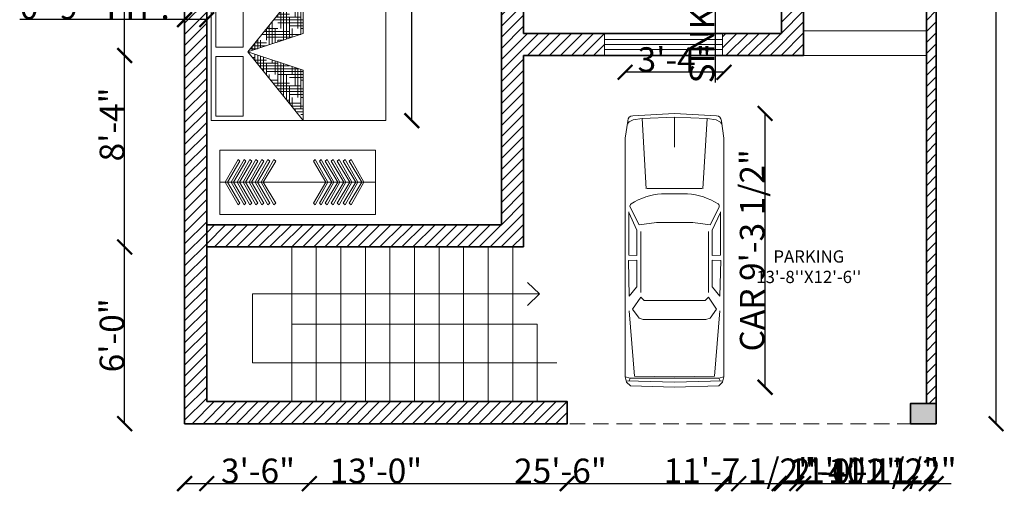
# Model space of a CAD drawing. Units: inches. Extents: x 1957 to 2456, y 1504 to 2088.
# Tile 1 of 6: x 1998 to 2399, y 1504 to 1703. Entities that reach past the tile are written whole.
import ezdxf

# ---------------------------------------------------------------- set-up
doc = ezdxf.new("R2010")
doc.units = ezdxf.units.IN
doc.header["$LTSCALE"] = 2
doc.linetypes.add('HIDDEN2', pattern=[4.7625, 3.175, -1.5875])
for name, color, linetype, lineweight in [('A-ANNO-DIMS', 2, 'Continuous', 18), ('A-ANNO-SYMB', 50, 'Continuous', 18), ('A-AREA-IDEN', 7, 'Continuous', 18), ('A-COLS', 12, 'Continuous', 35), ('A-COLS-PATT', 12, 'Continuous', 13), ('A-EQPM-VEHI', 8, 'Continuous', 18), ('A-FURN', 8, 'Continuous', 18), ('A-WALL-HIDN', 7, 'HIDDEN2', 18), ('A-WALL-PATT', 8, 'Continuous', 13), ('shelves', 204, 'Continuous', 18), ('Steps', 50, 'Continuous', 18), ('Walls', 7, 'Continuous', 35), ('Windows', 140, 'Continuous', 18)]:
    doc.layers.add(name, color=color, linetype=linetype, lineweight=lineweight)
doc.styles.get("Standard").update_dxf_attribs({"font": 'arial.ttf'})
doc.dimstyles.get("Standard").update_dxf_attribs({"dimtxt": 10, "dimasz": 6, "dimexe": 0.18, "dimexo": 0.0625, "dimgap": 0.09, "dimtad": 1, "dimdec": 1, "dimzin": 0, "dimdsep": 46, "dimlunit": 4, "dimtxsty": 'Standard', "dimblk": 'ARCHTICK', "dimcen": 0.09, "dimse1": 1, "dimse2": 1, "dimadec": 0, "dimazin": 0, "dimtfac": 1, "dimtdec": 1, "dimtofl": 0, "dimtmove": 0, "dimatfit": 3, "dimfxl": 1, "dimtolj": 1, "dimtzin": 0, "dimarcsym": 0})

# ---------------------------------------------------------------- blocks, each defined once
blk = doc.blocks.new('*X4')
at = {"color": 0}
for p, q in [((20.25, 14.812), (20.277, 14.812)), ((20.124, 14.688), (20.25, 14.688)), ((20.125, 14.5), (20.125, 14.689)), ((20.149, 14.719), (20.277, 14.719)), ((20.156, 14.625), (20.156, 14.728)), ((20.174, 14.75), (20.277, 14.75)), ((20.188, 14.75), (20.188, 14.767)), ((20.199, 14.781), (20.277, 14.781)), ((20.25, 14.319), (20.25, 14.75)), ((20.062, 14.257), (20.062, 14.612)), ((20.094, 14.375), (20.094, 14.65)), ((20.098, 14.656), (20.125, 14.656)), ((20.125, 14.594), (20.277, 14.594)), ((20.219, 14.309), (20.219, 14.625)), ((20.25, 14.625), (20.277, 14.625)), ((19.973, 14.5), (20.25, 14.5)), ((19.998, 14.531), (20.277, 14.531)), ((20, 14.237), (20, 14.5)), ((20.023, 14.562), (20.277, 14.562)), ((20.031, 14.247), (20.031, 14.573)), ((20.188, 14.299), (20.188, 14.5)), ((19.875, 14.25), (19.875, 14.379)), ((19.906, 14.375), (19.906, 14.417)), ((19.922, 14.438), (20, 14.438)), ((19.948, 14.469), (20.125, 14.469)), ((19.969, 14.226), (19.969, 14.375)), ((20, 14.375), (20.277, 14.375)), ((20.125, 14.406), (20.277, 14.406)), ((20.156, 14.288), (20.156, 14.375)), ((20.25, 14.438), (20.277, 14.438)), ((19.781, 14.164), (19.781, 14.262)), ((19.797, 14.281), (20.125, 14.281)), ((19.812, 14.174), (19.812, 14.301)), ((19.822, 14.312), (20.229, 14.312)), ((19.844, 14.185), (19.844, 14.34)), ((19.875, 14.344), (20.277, 14.344)), ((19.721, 14.188), (19.75, 14.188)), ((19.746, 14.219), (19.875, 14.219)), ((19.75, 14.154), (19.75, 14.223)), ((19.772, 14.25), (20, 14.25)), ((19.938, 14.216), (19.938, 14.25)), ((19.702, 14.094), (19.779, 14.094)), ((19.719, 14.073), (19.719, 14.114)), ((19.727, 14.062), (19.873, 14.062)), ((19.75, 14.034), (19.75, 14.103)), ((19.781, 13.995), (19.781, 14.093)), ((19.812, 14), (19.812, 14.082)), ((19.906, 13.84), (19.906, 14.051)), ((19.752, 14.031), (19.875, 14.031)), ((19.827, 13.938), (20.25, 13.938)), ((19.875, 13.878), (19.875, 14)), ((19.875, 13.969), (20.156, 13.969)), ((19.938, 13.801), (19.938, 14.041)), ((19.969, 13.875), (19.969, 14.031)), ((20, 14), (20, 14.02)), ((20, 14), (20.061, 14)), ((20.062, 13.645), (20.062, 14)), ((20.094, 13.625), (20.094, 13.989)), ((20.125, 13.75), (20.125, 13.979)), ((20.156, 13.875), (20.156, 13.969)), ((20.25, 13.5), (20.25, 13.937)), ((19.853, 13.906), (20.125, 13.906)), ((19.878, 13.875), (20, 13.875)), ((20.031, 13.684), (20.031, 13.875)), ((20.125, 13.844), (20.277, 13.844)), ((20.219, 13.451), (20.219, 13.875)), ((20.25, 13.875), (20.277, 13.875)), ((19.953, 13.781), (20.277, 13.781)), ((19.978, 13.75), (20.25, 13.75)), ((20, 13.812), (20.277, 13.812)), ((20, 13.723), (20, 13.75)), ((20.188, 13.49), (20.188, 13.75)), ((20.003, 13.719), (20.125, 13.719)), ((20.079, 13.625), (20.277, 13.625)), ((20.125, 13.656), (20.277, 13.656)), ((20.156, 13.529), (20.156, 13.625)), ((20.25, 13.688), (20.277, 13.688)), ((20.104, 13.594), (20.277, 13.594)), ((20.129, 13.562), (20.25, 13.562)), ((20.205, 13.469), (20.277, 13.469)), ((20.23, 13.438), (20.277, 13.438)), ((20.25, 13.5), (20.277, 13.5)), ((20.255, 13.406), (20.277, 13.406))]:
    blk.add_line(p, q, dxfattribs=at)
blk = doc.blocks.new('MAT-P13')
for p, q in [((-0.75, 0), (0.75, 0)), ((-0.75, 0), (-0.75, -1.9)), ((0.75, 0), (0.75, -1.9)), ((-0.7, -0.05), (-0.7, -0.35)), ((-0.7, -0.05), (-0.05, -0.05)), ((-0.05, -0.35), (-0.05, -0.05)), ((0.05, -0.05), (0.7, -0.05)), ((0.05, -0.35), (0.05, -0.05)), ((0.7, -0.05), (0.7, -0.35)), ((-0.75, -1.003), (0, -0.4)), ((0, -0.4), (-0.75, -1.003)), ((-0.7, -0.35), (-0.05, -0.35)), ((0, -0.4), (-0.2, -1.003)), ((0, -0.4), (0.2, -1.003)), ((0, -0.4), (0.75, -1.003)), ((0.05, -0.35), (0.7, -0.35)), ((-0.75, -1.003), (-0.2, -1.003)), ((0.2, -1.003), (0.75, -1.003)), ((0.75, -1.9), (-0.75, -1.9))]:
    blk.add_line(p, q)
at = {"xscale": -1, "rotation": 90}
blk.add_blockref('*X4', (14.128, 19.274), dxfattribs=at)
blk = doc.blocks.new('02PCAR12')
at = {"color": 0, "linetype": 'ByBlock'}
for p, q in [((-203, 38), (-207, 37)), ((-203, 38.08), (-204, 34.08)), ((-19, 38), (-203, 38)), ((-6, 36), (-19, 38)), ((-210, 34), (-211, 0)), ((-207, 37), (-210, 34)), ((-206, 37), (-207, 0)), ((-204, 34.08), (-206, 35.08)), ((-204, -34), (-204, 34)), ((-202.36, 30.78), (-203, 0)), ((-202.36, 30.78), (-152, 35)), ((-150.83, 32.3), (-157.9, 27.3)), ((-141.48, 25.99), (-150.83, 32.3)), ((-113.23, 35.5), (-140.79, 34.89)), ((-140.79, 34.89), (-133.96, 29.23)), ((-113, 29), (-113.23, 35.5)), ((-109.42, 29.02), (-109.19, 35.33)), ((-109.19, 35.33), (-75.91, 35.3)), ((-76.45, 35.3), (-90, 29)), ((-72.15, 34.24), (-85.91, 27.37)), ((-5, 32), (-6.45, 34.89)), ((-5, 32), (-4, 25)), ((0, 0), (-1.8, 32.21)), ((-157.9, 27.3), (-158.93, 24.08)), ((-158.93, 24.08), (-158.93, -24)), ((-141.48, 25.99), (-144.24, 23.52)), ((-144.24, 23.52), (-144.24, 0)), ((-91, 26), (-138, 26)), ((-134, 29), (-113, 29)), ((-90, 29), (-109.42, 29.02)), ((-58.25, 21.76), (-4, 25)), ((-4, 25), (-3, 0)), ((-58, 0), (-58, 21)), ((-84, -12), (-84, 12)), ((-62, 10), (-62, 0)), ((-210, -34), (-211, 0)), ((-206, -37), (-207, 0)), ((-202.36, -30.78), (-203, 0)), ((-144.24, -23.52), (-144.24, 0)), ((-62, -10), (-62, 0)), ((-58, 0), (-58, -21)), ((-3, 0), (-26, 0)), ((-4, -25), (-3, 0)), ((0, 0), (-1.8, -32.21)), ((-58.25, -21.76), (-4, -25)), ((-157.9, -27.3), (-158.93, -24.08)), ((-150.83, -32.3), (-157.9, -27.3)), ((-141.48, -25.99), (-150.83, -32.3)), ((-141.48, -25.99), (-144.24, -23.52)), ((-140.79, -34.89), (-133.96, -29.23)), ((-91, -26), (-138, -26)), ((-134, -29), (-113, -29)), ((-113, -29), (-113.23, -35.5)), ((-90, -29), (-109.42, -29.02)), ((-109.42, -29.02), (-109.19, -35.33)), ((-76.45, -35.3), (-90, -29)), ((-72.15, -34.24), (-85.91, -27.37)), ((-5, -32), (-4, -25)), ((-207, -37), (-210, -34)), ((-203, -38), (-207, -37)), ((-204, -34), (-206, -35)), ((-203, -38), (-204, -34)), ((-202.36, -30.69), (-152, -34.92)), ((-113.23, -35.5), (-140.79, -34.89)), ((-109.19, -35.33), (-75.91, -35.3)), ((-6, -36), (-19, -38)), ((-5, -32), (-6.45, -34.89)), ((-19, -38), (-203, -38))]:
    blk.add_line(p, q, dxfattribs=at)
for centre, radius, start, end in [((-71.36, 32.4), 2, 31.5638, 113.12574), ((-115.33, 5.39), 53.61, 4.93792, 31.5638), ((-8.24, 34), 2, 26.56505, 90), ((-5.8, 32), 4, 3.01279, 90), ((-461.05, -27.14), 379.08, 5.92644, 8.26698), ((-461.05, 27.14), 379.08, 351.73302, 354.07356), ((-115.33, -5.39), 53.61, 328.4362, 355.06208), ((-71.36, -32.4), 2, 246.87426, 328.4362), ((-8.24, -34), 2, 270, 333.43495), ((-5.8, -32), 4, 270, 356.98721)]:
    blk.add_arc(centre, radius, start, end, dxfattribs=at)
blk = doc.blocks.new('WIN-48IN')
for p, q in [((0, 6.5), (48, 6.5)), ((0, 4.5), (48, 4.5)), ((0, 2.5), (48, 2.5))]:
    blk.add_line(p, q)
blk.add_lwpolyline([(0, 9), (48, 9), (48, 0), (0, 0)], close=True)
blk = doc.blocks.new('WARDROBE-RAIL')
blk.add_line((0, 13.12), (63.46, 13.12))
blk.add_lwpolyline([(0, 26.23), (63.46, 26.23), (63.46, 0), (0, 0)], close=True)
for points in [[(2.25, 13.12), (7.43, 22.31), (8.16, 21.63), (3.1, 13.12)], [(4.68, 13.12), (9.87, 22.31), (10.6, 21.63), (5.54, 13.12)], [(7.12, 13.12), (12.3, 22.31), (13.03, 21.63), (7.98, 13.12)], [(9.56, 13.12), (14.74, 22.31), (15.47, 21.63), (10.41, 13.12)], [(11.99, 13.12), (17.18, 22.31), (17.91, 21.63), (12.85, 13.12)], [(14.43, 13.12), (19.61, 22.31), (20.34, 21.63), (15.29, 13.12)], [(16.87, 13.12), (22.05, 22.31), (22.78, 21.63), (17.72, 13.12)], [(44.01, 13.12), (38.82, 22.31), (38.09, 21.63), (43.15, 13.12)], [(46.44, 13.12), (41.26, 22.31), (40.53, 21.63), (45.59, 13.12)], [(48.88, 13.12), (43.7, 22.31), (42.96, 21.63), (48.02, 13.12)], [(51.31, 13.12), (46.13, 22.31), (45.4, 21.63), (50.46, 13.12)], [(53.75, 13.12), (48.57, 22.31), (47.84, 21.63), (52.89, 13.12)], [(56.19, 13.12), (51.01, 22.31), (50.27, 21.63), (55.33, 13.12)], [(58.62, 13.12), (53.44, 22.31), (52.71, 21.63), (57.77, 13.12)], [(2.25, 13.12), (7.43, 3.92), (8.16, 4.61), (3.1, 13.12)], [(4.68, 13.12), (9.87, 3.92), (10.6, 4.61), (5.54, 13.12)], [(7.12, 13.12), (12.3, 3.92), (13.03, 4.61), (7.98, 13.12)], [(9.56, 13.12), (14.74, 3.92), (15.47, 4.61), (10.41, 13.12)], [(11.99, 13.12), (17.18, 3.92), (17.91, 4.61), (12.85, 13.12)], [(14.43, 13.12), (19.61, 3.92), (20.34, 4.61), (15.29, 13.12)], [(16.87, 13.12), (22.05, 3.92), (22.78, 4.61), (17.72, 13.12)], [(44.01, 13.12), (38.82, 3.92), (38.09, 4.61), (43.15, 13.12)], [(46.44, 13.12), (41.26, 3.92), (40.53, 4.61), (45.59, 13.12)], [(48.88, 13.12), (43.7, 3.92), (42.96, 4.61), (48.02, 13.12)], [(51.31, 13.12), (46.13, 3.92), (45.4, 4.61), (50.46, 13.12)], [(53.75, 13.12), (48.57, 3.92), (47.84, 4.61), (52.89, 13.12)], [(56.19, 13.12), (51.01, 3.92), (50.27, 4.61), (55.33, 13.12)], [(58.62, 13.12), (53.44, 3.92), (52.71, 4.61), (57.77, 13.12)]]:
    blk.add_lwpolyline(points)
blk = doc.blocks.new('_ArchTick')
at = {"color": 0, "linetype": 'ByBlock', "const_width": 0.15}
blk.add_lwpolyline([(-0.5, -0.5), (0.5, 0.5)], dxfattribs=at)
blk = doc.blocks.new('*D24')
at = {"layer": 'A-ANNO-DIMS', "color": 0, "lineweight": -2, "transparency": 16777216}
for p, q in [((2065.03, 1702.85), (1997.9, 1702.85)), ((2074.03, 1702.85), (2065.03, 1702.85))]:
    blk.add_line(p, q, dxfattribs=at)
at = {"layer": 'Defpoints', "color": 0, "transparency": 16777216}
for p in [(2065.03, 1710.05), (2074.03, 1710.05), (2065.03, 1702.85)]:
    blk.add_point(p, dxfattribs=at)
at = {"layer": 'A-ANNO-DIMS', "color": 0, "lineweight": -2, "transparency": 16777216, "xscale": 6, "yscale": 6, "zscale": 6}
for p, rotation in [((2065.03, 1702.85), 179.9999999999986), ((2074.03, 1702.85), 359.9999999999986)]:
    blk.add_blockref('_ArchTick', p, dxfattribs=dict(at, rotation=rotation))
at = {"layer": 'A-ANNO-DIMS', "color": 0, "transparency": 16777216, "insert": (2028.47, 1708.05), "char_height": 10, "attachment_point": 5}
blk.add_mtext('\\A1;0\'-9" TYP.', dxfattribs=at)
blk = doc.blocks.new('*D30')
at = {"layer": 'A-ANNO-DIMS', "color": 0, "lineweight": -2, "transparency": 16777216}
for p, q in [((2157.56, 1717.76), (2157.56, 1785.3)), ((2157.56, 1661.68), (2157.56, 1717.76))]:
    blk.add_line(p, q, dxfattribs=at)
at = {"layer": 'Defpoints', "color": 0, "transparency": 16777216}
for p in [(2146.9, 1717.76), (2157.56, 1717.76), (2146.9, 1661.68)]:
    blk.add_point(p, dxfattribs=at)
at = {"layer": 'A-ANNO-DIMS', "color": 0, "lineweight": -2, "transparency": 16777216, "xscale": 6, "yscale": 6, "zscale": 6}
for p, rotation in [((2157.56, 1717.76), 90), ((2157.56, 1661.68), 270)]:
    blk.add_blockref('_ArchTick', p, dxfattribs=dict(at, rotation=rotation))
at = {"layer": 'A-ANNO-DIMS', "color": 0, "transparency": 16777216, "insert": (2152.36, 1754.53), "char_height": 10, "attachment_point": 5, "rotation": 90}
blk.add_mtext('\\A1;4\'-8" TYP.', dxfattribs=at)
blk = doc.blocks.new('*D41')
at = {"layer": 'A-ANNO-DIMS', "color": 0, "lineweight": -2, "transparency": 16777216}
for p, q in [((2281, 1801.1), (2281, 1777.56)), ((2281, 1777.56), (2281, 1677.29))]:
    blk.add_line(p, q, dxfattribs=at)
at = {"layer": 'Defpoints', "color": 0, "transparency": 16777216}
for p in [(2284.53, 1801.1), (2281, 1777.56), (2284.53, 1777.56)]:
    blk.add_point(p, dxfattribs=at)
at = {"layer": 'A-ANNO-DIMS', "color": 0, "lineweight": -2, "transparency": 16777216, "xscale": 6, "yscale": 6, "zscale": 6}
for p, rotation in [((2281, 1801.1), 90), ((2281, 1777.56), 270)]:
    blk.add_blockref('_ArchTick', p, dxfattribs=dict(at, rotation=rotation))
at = {"layer": 'A-ANNO-DIMS', "color": 0, "transparency": 16777216, "insert": (2275.74, 1724.42), "char_height": 10, "attachment_point": 5, "rotation": 90}
blk.add_mtext('\\A1;SINK 1\'-11 1/2"', dxfattribs=at)
blk = doc.blocks.new('*D43')
at = {"layer": 'A-ANNO-DIMS', "color": 0, "lineweight": -2, "transparency": 16777216}
blk.add_line((2301.35, 1553.07), (2301.35, 1664.66), dxfattribs=at)
at = {"layer": 'Defpoints', "color": 0, "transparency": 16777216}
for p in [(2284.62, 1664.66), (2301.35, 1664.66), (2284.62, 1553.07)]:
    blk.add_point(p, dxfattribs=at)
at = {"layer": 'A-ANNO-DIMS', "color": 0, "lineweight": -2, "transparency": 16777216, "xscale": 6, "yscale": 6, "zscale": 6}
for p, rotation in [((2301.35, 1664.66), 90), ((2301.35, 1553.07), 270)]:
    blk.add_blockref('_ArchTick', p, dxfattribs=dict(at, rotation=rotation))
at = {"layer": 'A-ANNO-DIMS', "color": 0, "transparency": 16777216, "insert": (2296.09, 1608.86), "char_height": 10, "attachment_point": 5, "rotation": 90}
blk.add_mtext('\\A1;CAR 9\'-3 1/2"', dxfattribs=at)
blk = doc.blocks.new('*D44')
at = {"layer": 'A-ANNO-DIMS', "color": 0, "lineweight": -2, "transparency": 16777216}
blk.add_line((2284.62, 1681.39), (2244.38, 1681.39), dxfattribs=at)
at = {"layer": 'Defpoints', "color": 0, "transparency": 16777216}
for p in [(2244.38, 1681.39), (2244.38, 1664.66), (2284.62, 1664.66)]:
    blk.add_point(p, dxfattribs=at)
at = {"layer": 'A-ANNO-DIMS', "color": 0, "lineweight": -2, "transparency": 16777216, "xscale": 6, "yscale": 6, "zscale": 6, "rotation": 180}
blk.add_blockref('_ArchTick', (2244.38, 1681.39), dxfattribs=at)
at = {"layer": 'A-ANNO-DIMS', "color": 0, "lineweight": -2, "transparency": 16777216, "xscale": 6, "yscale": 6, "zscale": 6}
blk.add_blockref('_ArchTick', (2284.62, 1681.39), dxfattribs=at)
at = {"layer": 'A-ANNO-DIMS', "color": 0, "transparency": 16777216, "insert": (2264.5, 1686.59), "char_height": 10, "attachment_point": 5}
blk.add_mtext('\\A1;3\'-4"', dxfattribs=at)
blk = doc.blocks.new('*D45')
at = {"layer": 'A-ANNO-DIMS', "color": 0, "lineweight": -2, "transparency": 16777216}
blk.add_line((2065.03, 1513.82), (2371.03, 1513.82), dxfattribs=at)
at = {"layer": 'Defpoints', "color": 0, "transparency": 16777216}
for p in [(2065.03, 1538.22), (2371.03, 1538.22), (2371.03, 1513.82)]:
    blk.add_point(p, dxfattribs=at)
at = {"layer": 'A-ANNO-DIMS', "color": 0, "lineweight": -2, "transparency": 16777216, "xscale": 6, "yscale": 6, "zscale": 6, "rotation": 180}
blk.add_blockref('_ArchTick', (2065.03, 1513.82), dxfattribs=at)
at = {"layer": 'A-ANNO-DIMS', "color": 0, "lineweight": -2, "transparency": 16777216, "xscale": 6, "yscale": 6, "zscale": 6}
blk.add_blockref('_ArchTick', (2371.03, 1513.82), dxfattribs=at)
at = {"layer": 'A-ANNO-DIMS', "color": 0, "transparency": 16777216, "insert": (2218.03, 1519.01), "char_height": 10, "attachment_point": 5}
blk.add_mtext('\\A1;25\'-6"', dxfattribs=at)
blk = doc.blocks.new('*D46')
at = {"layer": 'A-ANNO-DIMS', "color": 0, "lineweight": -2, "transparency": 16777216}
blk.add_line((2395.43, 1538.22), (2395.43, 2021.22), dxfattribs=at)
at = {"layer": 'Defpoints', "color": 0, "transparency": 16777216}
for p in [(2371.03, 2021.22), (2395.43, 2021.22), (2371.03, 1538.22)]:
    blk.add_point(p, dxfattribs=at)
at = {"layer": 'A-ANNO-DIMS', "color": 0, "lineweight": -2, "transparency": 16777216, "xscale": 6, "yscale": 6, "zscale": 6}
for p, rotation in [((2395.43, 2021.22), 90), ((2395.43, 1538.22), 270)]:
    blk.add_blockref('_ArchTick', p, dxfattribs=dict(at, rotation=rotation))
at = {"layer": 'A-ANNO-DIMS', "color": 0, "transparency": 16777216, "insert": (2390.23, 1779.72), "char_height": 10, "attachment_point": 5, "rotation": 90}
blk.add_mtext('\\A1;40\'-3"', dxfattribs=at)
blk = doc.blocks.new('*D51')
at = {"layer": 'A-ANNO-DIMS', "color": 0, "lineweight": -2, "transparency": 16777216}
blk.add_line((2040.63, 1538.22), (2040.63, 1610.22), dxfattribs=at)
at = {"layer": 'Defpoints', "color": 0, "transparency": 16777216}
for p in [(2040.63, 1610.22), (2074.03, 1610.22), (2065.03, 1538.22)]:
    blk.add_point(p, dxfattribs=at)
at = {"layer": 'A-ANNO-DIMS', "color": 0, "lineweight": -2, "transparency": 16777216, "xscale": 6, "yscale": 6, "zscale": 6}
for p, rotation in [((2040.63, 1610.22), 90), ((2040.63, 1538.22), 270)]:
    blk.add_blockref('_ArchTick', p, dxfattribs=dict(at, rotation=rotation))
at = {"layer": 'A-ANNO-DIMS', "color": 0, "transparency": 16777216, "insert": (2035.44, 1574.22), "char_height": 10, "attachment_point": 5, "rotation": 90}
blk.add_mtext('\\A1;6\'-0"', dxfattribs=at)
blk = doc.blocks.new('*D52')
at = {"layer": 'A-ANNO-DIMS', "color": 0, "lineweight": -2, "transparency": 16777216}
blk.add_line((2040.63, 1610.22), (2040.63, 1710.05), dxfattribs=at)
at = {"layer": 'Defpoints', "color": 0, "transparency": 16777216}
for p in [(2040.63, 1710.05), (2074.03, 1710.05), (2074.03, 1610.22)]:
    blk.add_point(p, dxfattribs=at)
at = {"layer": 'A-ANNO-DIMS', "color": 0, "lineweight": -2, "transparency": 16777216, "xscale": 6, "yscale": 6, "zscale": 6}
for p, rotation in [((2040.63, 1710.05), 90), ((2040.63, 1610.22), 270)]:
    blk.add_blockref('_ArchTick', p, dxfattribs=dict(at, rotation=rotation))
at = {"layer": 'A-ANNO-DIMS', "color": 0, "transparency": 16777216, "insert": (2035.44, 1660.14), "char_height": 10, "attachment_point": 5, "rotation": 90}
blk.add_mtext('\\A1;8\'-4"', dxfattribs=at)
blk = doc.blocks.new('*D53')
at = {"layer": 'A-ANNO-DIMS', "color": 0, "lineweight": -2, "transparency": 16777216}
blk.add_line((2065.03, 1513.82), (2220.79, 1513.82), dxfattribs=at)
at = {"layer": 'Defpoints', "color": 0, "transparency": 16777216}
for p in [(2065.03, 1538.22), (2220.79, 1538.22), (2220.79, 1513.82)]:
    blk.add_point(p, dxfattribs=at)
at = {"layer": 'A-ANNO-DIMS', "color": 0, "lineweight": -2, "transparency": 16777216, "xscale": 6, "yscale": 6, "zscale": 6, "rotation": 180}
blk.add_blockref('_ArchTick', (2065.03, 1513.82), dxfattribs=at)
at = {"layer": 'A-ANNO-DIMS', "color": 0, "lineweight": -2, "transparency": 16777216, "xscale": 6, "yscale": 6, "zscale": 6}
blk.add_blockref('_ArchTick', (2220.79, 1513.82), dxfattribs=at)
at = {"layer": 'A-ANNO-DIMS', "color": 0, "transparency": 16777216, "insert": (2142.91, 1519.02), "char_height": 10, "attachment_point": 5}
blk.add_mtext('\\A1;13\'-0"', dxfattribs=at)
blk = doc.blocks.new('*D54')
at = {"layer": 'A-ANNO-DIMS', "color": 0, "lineweight": -2, "transparency": 16777216}
blk.add_line((2220.79, 1513.82), (2360.54, 1513.82), dxfattribs=at)
at = {"layer": 'Defpoints', "color": 0, "transparency": 16777216}
for p in [(2220.79, 1538.22), (2360.54, 1538.22), (2360.54, 1513.82)]:
    blk.add_point(p, dxfattribs=at)
at = {"layer": 'A-ANNO-DIMS', "color": 0, "lineweight": -2, "transparency": 16777216, "xscale": 6, "yscale": 6, "zscale": 6, "rotation": 180}
blk.add_blockref('_ArchTick', (2220.79, 1513.82), dxfattribs=at)
at = {"layer": 'A-ANNO-DIMS', "color": 0, "lineweight": -2, "transparency": 16777216, "xscale": 6, "yscale": 6, "zscale": 6}
blk.add_blockref('_ArchTick', (2360.54, 1513.82), dxfattribs=at)
at = {"layer": 'A-ANNO-DIMS', "color": 0, "transparency": 16777216, "insert": (2290.66, 1519.08), "char_height": 10, "attachment_point": 5}
blk.add_mtext('\\A1;11\'-7 1/2"', dxfattribs=at)
blk = doc.blocks.new('*D55')
at = {"layer": 'A-ANNO-DIMS', "color": 0, "lineweight": -2, "transparency": 16777216}
blk.add_line((2317.03, 1513.82), (2367.03, 1513.82), dxfattribs=at)
at = {"layer": 'Defpoints', "color": 0, "transparency": 16777216}
for p in [(2317.03, 1688.22), (2367.03, 1688.22), (2367.03, 1513.82)]:
    blk.add_point(p, dxfattribs=at)
at = {"layer": 'A-ANNO-DIMS', "color": 0, "lineweight": -2, "transparency": 16777216, "xscale": 6, "yscale": 6, "zscale": 6, "rotation": 180}
blk.add_blockref('_ArchTick', (2317.03, 1513.82), dxfattribs=at)
at = {"layer": 'A-ANNO-DIMS', "color": 0, "lineweight": -2, "transparency": 16777216, "xscale": 6, "yscale": 6, "zscale": 6}
blk.add_blockref('_ArchTick', (2367.03, 1513.82), dxfattribs=at)
at = {"layer": 'A-ANNO-DIMS', "color": 0, "transparency": 16777216, "insert": (2342.03, 1518.93), "char_height": 10, "attachment_point": 5}
blk.add_mtext('\\A1;4\'-2"', dxfattribs=at)
blk = doc.blocks.new('*D56')
at = {"layer": 'A-ANNO-DIMS', "color": 0, "lineweight": -2, "transparency": 16777216}
blk.add_line((2040.63, 1688.22), (2040.63, 1869.22), dxfattribs=at)
at = {"layer": 'Defpoints', "color": 0, "transparency": 16777216}
for p in [(2040.63, 1869.22), (2367.03, 1869.22), (2367.03, 1688.22)]:
    blk.add_point(p, dxfattribs=at)
at = {"layer": 'A-ANNO-DIMS', "color": 0, "lineweight": -2, "transparency": 16777216, "xscale": 6, "yscale": 6, "zscale": 6}
for p, rotation in [((2040.63, 1869.22), 90), ((2040.63, 1688.22), 270)]:
    blk.add_blockref('_ArchTick', p, dxfattribs=dict(at, rotation=rotation))
at = {"layer": 'A-ANNO-DIMS', "color": 0, "transparency": 16777216, "insert": (2035.44, 1778.72), "char_height": 10, "attachment_point": 5, "rotation": 90}
blk.add_mtext('\\A1;15\'-1"', dxfattribs=at)
blk = doc.blocks.new('*D59')
at = {"layer": 'A-ANNO-DIMS', "color": 0, "lineweight": -2, "transparency": 16777216}
blk.add_line((2074.03, 1513.82), (2115.8, 1513.82), dxfattribs=at)
at = {"layer": 'Defpoints', "color": 0, "transparency": 16777216}
for p in [(2074.03, 1760.22), (2115.8, 1760.22), (2115.8, 1513.82)]:
    blk.add_point(p, dxfattribs=at)
at = {"layer": 'A-ANNO-DIMS', "color": 0, "lineweight": -2, "transparency": 16777216, "xscale": 6, "yscale": 6, "zscale": 6, "rotation": 180}
blk.add_blockref('_ArchTick', (2074.03, 1513.82), dxfattribs=at)
at = {"layer": 'A-ANNO-DIMS', "color": 0, "lineweight": -2, "transparency": 16777216, "xscale": 6, "yscale": 6, "zscale": 6}
blk.add_blockref('_ArchTick', (2115.8, 1513.82), dxfattribs=at)
at = {"layer": 'A-ANNO-DIMS', "color": 0, "transparency": 16777216, "insert": (2094.91, 1519.02), "char_height": 10, "attachment_point": 5}
blk.add_mtext('\\A1;3\'-6"', dxfattribs=at)
blk = doc.blocks.new('*D60')
at = {"layer": 'A-ANNO-DIMS', "color": 0, "lineweight": -2, "transparency": 16777216}
for p, q in [((2284.03, 1513.82), (2308.03, 1513.82)), ((2308.03, 1513.82), (2340.97, 1513.82))]:
    blk.add_line(p, q, dxfattribs=at)
at = {"layer": 'Defpoints', "color": 0, "transparency": 16777216}
for p in [(2308.03, 1697.22), (2284.03, 1688.22), (2308.03, 1513.82)]:
    blk.add_point(p, dxfattribs=at)
at = {"layer": 'A-ANNO-DIMS', "color": 0, "lineweight": -2, "transparency": 16777216, "xscale": 6, "yscale": 6, "zscale": 6, "rotation": 180}
blk.add_blockref('_ArchTick', (2284.03, 1513.82), dxfattribs=at)
at = {"layer": 'A-ANNO-DIMS', "color": 0, "lineweight": -2, "transparency": 16777216, "xscale": 6, "yscale": 6, "zscale": 6}
blk.add_blockref('_ArchTick', (2308.03, 1513.82), dxfattribs=at)
at = {"layer": 'A-ANNO-DIMS', "color": 0, "transparency": 16777216, "insert": (2327.5, 1519.01), "char_height": 10, "attachment_point": 5}
blk.add_mtext('\\A1;2\'-0"', dxfattribs=at)
blk = doc.blocks.new('*D62')
at = {"layer": 'A-ANNO-DIMS', "color": 0, "lineweight": -2, "transparency": 16777216}
for p, q in [((2074.03, 2045.62), (2108.63, 2045.62)), ((2108.63, 2045.62), (2172.63, 2045.62))]:
    blk.add_line(p, q, dxfattribs=at)
at = {"layer": 'Defpoints', "color": 0, "transparency": 16777216}
for p in [(2108.63, 2045.62), (2074.03, 1547.22), (2108.63, 1547.22)]:
    blk.add_point(p, dxfattribs=at)
at = {"layer": 'A-ANNO-DIMS', "color": 0, "lineweight": -2, "transparency": 16777216, "xscale": 6, "yscale": 6, "zscale": 6, "rotation": 180}
blk.add_blockref('_ArchTick', (2074.03, 2045.62), dxfattribs=at)
at = {"layer": 'A-ANNO-DIMS', "color": 0, "lineweight": -2, "transparency": 16777216, "xscale": 6, "yscale": 6, "zscale": 6}
blk.add_blockref('_ArchTick', (2108.63, 2045.62), dxfattribs=at)
at = {"layer": 'A-ANNO-DIMS', "color": 0, "transparency": 16777216, "insert": (2143.63, 2050.88), "char_height": 10, "attachment_point": 5}
blk.add_mtext('\\A1;2\'-10 1/2"', dxfattribs=at)
blk = doc.blocks.new('*D63')
at = {"layer": 'A-ANNO-DIMS', "color": 0, "lineweight": -2, "transparency": 16777216}
for p, q in [((2108.63, 2045.62), (2118.63, 2045.62)), ((2118.63, 2045.62), (2159.16, 2045.62))]:
    blk.add_line(p, q, dxfattribs=at)
at = {"layer": 'Defpoints', "color": 0, "transparency": 16777216}
for p in [(2118.63, 2045.62), (2108.63, 1547.22), (2118.63, 1547.22)]:
    blk.add_point(p, dxfattribs=at)
at = {"layer": 'A-ANNO-DIMS', "color": 0, "lineweight": -2, "transparency": 16777216, "xscale": 6, "yscale": 6, "zscale": 6, "rotation": 180}
blk.add_blockref('_ArchTick', (2108.63, 2045.62), dxfattribs=at)
at = {"layer": 'A-ANNO-DIMS', "color": 0, "lineweight": -2, "transparency": 16777216, "xscale": 6, "yscale": 6, "zscale": 6}
blk.add_blockref('_ArchTick', (2118.63, 2045.62), dxfattribs=at)
at = {"layer": 'A-ANNO-DIMS', "color": 0, "transparency": 16777216, "insert": (2141.89, 2050.81), "char_height": 10, "attachment_point": 5}
blk.add_mtext('\\A1;0\'-10"', dxfattribs=at)
blk = doc.blocks.new('*D64')
at = {"layer": 'A-ANNO-DIMS', "color": 0, "lineweight": -2, "transparency": 16777216}
for p, q in [((2290.6, 1513.82), (2314.26, 1513.82)), ((2314.26, 1513.82), (2377.15, 1513.82))]:
    blk.add_line(p, q, dxfattribs=at)
at = {"layer": 'Defpoints', "color": 0, "transparency": 16777216}
for p in [(2290.6, 1933.88), (2314.26, 1933.88), (2314.26, 1513.82)]:
    blk.add_point(p, dxfattribs=at)
at = {"layer": 'A-ANNO-DIMS', "color": 0, "lineweight": -2, "transparency": 16777216, "xscale": 6, "yscale": 6, "zscale": 6, "rotation": 180}
blk.add_blockref('_ArchTick', (2290.6, 1513.82), dxfattribs=at)
at = {"layer": 'A-ANNO-DIMS', "color": 0, "lineweight": -2, "transparency": 16777216, "xscale": 6, "yscale": 6, "zscale": 6}
blk.add_blockref('_ArchTick', (2314.26, 1513.82), dxfattribs=at)
at = {"layer": 'A-ANNO-DIMS', "color": 0, "transparency": 16777216, "insert": (2348.71, 1519.08), "char_height": 10, "attachment_point": 5}
blk.add_mtext('\\A1;1\'-11 1/2"', dxfattribs=at)
blk = doc.blocks.new('*D66')
at = {"layer": 'A-ANNO-DIMS', "color": 0, "lineweight": -2, "transparency": 16777216}
for p, q in [((2284.61, 1513.82), (2307.13, 1513.82)), ((2307.13, 1513.82), (2370.02, 1513.82))]:
    blk.add_line(p, q, dxfattribs=at)
at = {"layer": 'Defpoints', "color": 0, "transparency": 16777216}
for p in [(2284.61, 1737.54), (2307.13, 1737.54), (2307.13, 1513.82)]:
    blk.add_point(p, dxfattribs=at)
at = {"layer": 'A-ANNO-DIMS', "color": 0, "lineweight": -2, "transparency": 16777216, "xscale": 6, "yscale": 6, "zscale": 6, "rotation": 180}
blk.add_blockref('_ArchTick', (2284.61, 1513.82), dxfattribs=at)
at = {"layer": 'A-ANNO-DIMS', "color": 0, "lineweight": -2, "transparency": 16777216, "xscale": 6, "yscale": 6, "zscale": 6}
blk.add_blockref('_ArchTick', (2307.13, 1513.82), dxfattribs=at)
at = {"layer": 'A-ANNO-DIMS', "color": 0, "transparency": 16777216, "insert": (2341.58, 1519.08), "char_height": 10, "attachment_point": 5}
blk.add_mtext('\\A1;1\'-10 1/2"', dxfattribs=at)

msp = doc.modelspace()

# ---------------------------------------------------------------- hatches: boundary and pattern name
at = {"layer": 'A-COLS-PATT'}
h = msp.add_hatch(color=256, dxfattribs=at)
h.dxf.hatch_style = 1
h.paths.add_polyline_path([(2367.03, 1546.41), (2360.54, 1546.41), (2360.54, 1538.22), (2367.03, 1538.22)])
h.paths.add_polyline_path([(2371.03, 1546.41), (2367.03, 1546.41), (2367.03, 1538.22), (2371.03, 1538.22)])
at = {"layer": 'A-WALL-PATT', "transparency": 33554585}
h = msp.add_hatch(dxfattribs=at)
h.set_pattern_fill('ANSI31', color=256)
h.paths.add_polyline_path([(2129.18, 2021.22), (2065.03, 2021.22), (2065.03, 1857.22), (2074.03, 1857.22), (2074.03, 1869.22), (2115.8, 1869.22), (2115.8, 1878.22), (2074.03, 1878.22), (2074.03, 2012.22), (2129.18, 2012.22)])
h.paths.add_polyline_path([(2209.75, 2021.22), (2189.18, 2021.22), (2189.18, 2012.22), (2194.03, 2012.22), (2194.03, 1878.22), (2190.56, 1878.22), (2190.56, 1869.22), (2203.03, 1869.22), (2203.03, 2012.22), (2209.75, 2012.22)])
h.paths.add_polyline_path([(2273.18, 2021.22), (2245.68, 2021.22), (2245.68, 2012.22), (2273.18, 2012.22)])
h.paths.add_polyline_path([(2371.03, 2021.22), (2333.18, 2021.22), (2333.18, 2012.22), (2362.03, 2012.22), (2362.03, 1968.25), (2371.03, 1968.25)])
h.paths.add_polyline_path([(2371.03, 1869.22), (2367.03, 1869.22), (2367.03, 1546.41), (2371.03, 1546.41)])
h.paths.add_polyline_path([(2317.03, 1820.22), (2247.38, 1820.22), (2247.38, 1811.22), (2308.03, 1811.22), (2308.03, 1697.22), (2284.03, 1697.22), (2284.03, 1688.22), (2317.03, 1688.22)])
h.paths.add_polyline_path([(2236.03, 1697.22), (2203.03, 1697.22), (2203.03, 1811.22), (2211.8, 1811.22), (2211.8, 1820.22), (2194.03, 1820.22), (2194.03, 1619.22), (2074.03, 1619.22), (2074.03, 1610.22), (2203.03, 1610.22), (2203.03, 1688.22), (2236.03, 1688.22)])
h.paths.add_polyline_path([(2153.03, 1869.22), (2155.49, 1869.22), (2155.49, 1877.47), (2155.49, 1878.22), (2146.03, 1878.22), (2146.03, 1871.1), (2146.03, 1869.22), (2149.03, 1869.22), (2149.03, 1821.22), (2074.03, 1821.22), (2074.03, 1833.22), (2065.03, 1833.22), (2065.03, 1805.22), (2074.03, 1805.22), (2074.03, 1817.22), (2149.03, 1817.22), (2149.03, 1769.22), (2146.03, 1769.22), (2146.03, 1760.22), (2153.03, 1760.22), (2156.02, 1760.22), (2156.02, 1760.87), (2156.02, 1769.11), (2153.03, 1769.11)])
h.paths.add_polyline_path([(2074.03, 1781.22), (2065.03, 1781.22), (2065.03, 1758.05), (2074.03, 1758.05), (2074.03, 1760.22), (2115.8, 1760.22), (2115.8, 1767.33), (2115.8, 1769.22), (2074.03, 1769.22)])
h = msp.add_hatch(dxfattribs=at)
h.set_pattern_fill('ANSI31', color=256)
h.paths.add_polyline_path([(2371.03, 1920.25), (2362.03, 1920.25), (2362.03, 1878.22), (2308.03, 1878.22), (2308.03, 1869.22), (2308.03, 1856.15), (2317.03, 1856.15), (2317.03, 1869.22), (2371.03, 1869.22)])
h.paths.add_polyline_path([(2074.03, 1710.05), (2065.03, 1710.05), (2065.03, 1538.22), (2203.03, 1538.22), (2220.79, 1538.22), (2220.79, 1547.22), (2203.03, 1547.22), (2074.03, 1547.22)])

# ---------------------------------------------------------------- linework, layer by layer
at = {"layer": 'A-ANNO-SYMB'}
for p, q in [((2092.7, 1562.97), (2092.7, 1591.08)), ((2092.7, 1591.08), (2209.54, 1591.08)), ((2216.62, 1562.97), (2092.7, 1562.97))]:
    msp.add_line(p, q, dxfattribs=at)
msp.add_lwpolyline([(2204.59, 1586.37), (2209.54, 1591.08), (2204.59, 1595.79)], dxfattribs=at)
at = {"layer": 'A-COLS'}
msp.add_lwpolyline([(2371.03, 1538.22), (2360.54, 1538.22), (2360.54, 1546.41), (2371.03, 1546.41)], close=True, dxfattribs=at)
at = {"layer": 'A-WALL-HIDN'}
msp.add_line((2371.03, 1538.22), (2220.79, 1538.22), dxfattribs=at)
at = {"layer": 'Steps'}
for p, q in [((2317.03, 1698.22), (2367.03, 1698.22)), ((2317.03, 1688.22), (2367.03, 1688.22)), ((2108.63, 1610.22), (2108.63, 1547.22)), ((2118.63, 1610.22), (2118.63, 1547.22)), ((2128.63, 1610.22), (2128.63, 1547.22)), ((2138.63, 1610.22), (2138.63, 1547.22)), ((2148.63, 1610.22), (2148.63, 1547.22)), ((2158.63, 1610.22), (2158.63, 1547.22)), ((2168.63, 1610.22), (2168.63, 1547.22)), ((2178.63, 1610.22), (2178.63, 1547.22)), ((2188.63, 1610.22), (2188.63, 1547.22)), ((2198.63, 1610.22), (2198.63, 1547.22)), ((2198.63, 1578.72), (2108.63, 1578.72)), ((2198.63, 1578.72), (2208.63, 1578.72)), ((2208.63, 1578.72), (2208.63, 1547.22))]:
    msp.add_line(p, q, dxfattribs=at)
at = {"layer": 'Walls'}
for p, q in [((2065.03, 2021.22), (2065.03, 1538.22)), ((2371.03, 2021.22), (2371.03, 1538.22)), ((2367.03, 1869.22), (2367.03, 1546.41)), ((2194.03, 1820.22), (2194.03, 1619.22)), ((2317.03, 1820.22), (2317.03, 1688.22)), ((2203.03, 1811.22), (2203.03, 1697.22)), ((2308.03, 1811.22), (2308.03, 1697.22)), ((2074.03, 1760.22), (2074.03, 1547.22)), ((2308.03, 1697.22), (2203.03, 1697.22)), ((2317.03, 1688.22), (2203.03, 1688.22)), ((2203.03, 1688.22), (2203.03, 1610.22)), ((2194.03, 1619.22), (2074.03, 1619.22)), ((2203.03, 1610.22), (2074.03, 1610.22))]:
    msp.add_line(p, q, dxfattribs=at)
msp.add_lwpolyline([(2065.03, 1538.22), (2203.03, 1538.22), (2220.79, 1538.22), (2220.79, 1547.22), (2203.03, 1547.22), (2074.03, 1547.22)], dxfattribs=at)

# ---------------------------------------------------------------- block references
at = {"layer": 'A-EQPM-VEHI', "xscale": 0.5288402406434952, "yscale": 0.5288402406434952, "zscale": 0.5288402406434952, "rotation": 90}
msp.add_blockref('02PCAR12', (2264.52, 1664.66), dxfattribs=at)
at = {"layer": 'A-FURN', "xscale": 37.39052698416379, "yscale": 37.39052698416379, "zscale": 37.39052698416379, "rotation": 90}
msp.add_blockref('MAT-P13', (2075.86, 1689.72), dxfattribs=at)
at = {"layer": 'shelves'}
msp.add_blockref('WARDROBE-RAIL', (2079.36, 1623.49), dxfattribs=at)
at = {"layer": 'Windows'}
msp.add_blockref('WIN-48IN', (2236.03, 1688.22), dxfattribs=at)

# ---------------------------------------------------------------- texts
at = {"layer": 'A-AREA-IDEN', "insert": (2293.08, 1608.85), "char_height": 5, "attachment_point": 1}
msp.add_mtext_dynamic_manual_height_columns("\\pxqc;PARKING\\P13'-8''X12'-6''", width=52.1707, gutter_width=12.5, heights=[0], dxfattribs=at)

# ---------------------------------------------------------------- dimensions: what is measured, and where the dimension line sits
at = {"layer": 'A-ANNO-DIMS'}
for base, p1, p2, picture, middle in [((2108.63, 2045.62), (2074.03, 1547.22), (2108.63, 1547.22), '*D62', (2143.63, 2050.88)), ((2118.63, 2045.62), (2108.63, 1547.22), (2118.63, 1547.22), '*D63', (2141.89, 2050.81)), ((2314.26, 1513.82), (2290.6, 1933.88), (2314.26, 1933.88), '*D64', (2348.71, 1519.08)), ((2115.8, 1513.82), (2074.03, 1760.22), (2115.8, 1760.22), '*D59', (2094.91, 1519.02)), ((2307.13, 1513.82), (2284.61, 1737.54), (2307.13, 1737.54), '*D66', (2341.58, 1519.08)), ((2308.03, 1513.82), (2284.03, 1688.22), (2308.03, 1697.22), '*D60', (2327.5, 1519.01)), ((2367.03, 1513.82), (2317.03, 1688.22), (2367.03, 1688.22), '*D55', (2342.03, 1518.93)), ((2371.03, 1513.82), (2065.03, 1538.22), (2371.03, 1538.22), '*D45', (2218.03, 1519.01)), ((2220.79, 1513.82), (2065.03, 1538.22), (2220.79, 1538.22), '*D53', (2142.91, 1519.02)), ((2360.5368, 1513.8189), (2220.7922, 1538.2189), (2360.5368, 1538.2189), '*D54', (2290.6645, 1519.0794))]:
    dim = msp.add_linear_dim(base=base, p1=p1, p2=p2, dimstyle='Standard', override={"dimdec": 1, "dimlfac": 1, "dimrnd": 0, "dimzin": 1, "dimdsep": 46, "dimlunit": 4, "dimfrac": 2}, dxfattribs=at)
    dim.commit()
    dim.dimension.update_dxf_attribs({"geometry": picture, "text_midpoint": middle})
for base, p1, p2, angle, picture, middle in [((2395.43, 2021.22), (2371.03, 1538.22), (2371.03, 2021.22), 90, '*D46', (2390.23, 1779.72)), ((2040.63, 1869.22), (2367.03, 1688.22), (2367.03, 1869.22), 90, '*D56', (2035.44, 1778.72)), ((2040.63, 1710.05), (2074.03, 1610.22), (2074.03, 1710.05), 90, '*D52', (2035.44, 1660.14)), ((2244.38, 1681.39), (2284.62, 1664.66), (2244.38, 1664.66), 180, '*D44', (2264.5, 1686.59)), ((2040.63, 1610.22), (2065.03, 1538.22), (2074.03, 1610.22), 90, '*D51', (2035.44, 1574.22))]:
    dim = msp.add_linear_dim(base=base, p1=p1, p2=p2, angle=angle, dimstyle='Standard', override={"dimdec": 1, "dimlfac": 1, "dimrnd": 0, "dimzin": 1, "dimdsep": 46, "dimlunit": 4, "dimfrac": 2}, dxfattribs=at)
    dim.commit()
    dim.dimension.update_dxf_attribs({"geometry": picture, "text_midpoint": middle})
for base, p1, p2, angle, text, picture, middle in [((2281, 1777.56), (2284.53, 1801.1), (2284.53, 1777.56), 270, 'SINK <>', '*D41', (2275.74, 1724.42)), ((2157.56, 1717.76), (2146.9, 1661.68), (2146.9, 1717.76), 90, '<> TYP.', '*D30', (2152.36, 1754.53)), ((2065.03, 1702.85), (2074.03, 1710.05), (2065.03, 1710.05), 180, '<> TYP.', '*D24', (2028.47, 1708.05)), ((2301.35, 1664.66), (2284.62, 1553.07), (2284.62, 1664.66), 90, 'CAR <>', '*D43', (2296.09, 1608.86))]:
    dim = msp.add_linear_dim(base=base, p1=p1, p2=p2, angle=angle, text=text, dimstyle='Standard', override={"dimdec": 1, "dimlfac": 1, "dimrnd": 0, "dimzin": 1, "dimdsep": 46, "dimlunit": 4, "dimfrac": 2}, dxfattribs=at)
    dim.commit()
    dim.dimension.update_dxf_attribs({"geometry": picture, "text_midpoint": middle})

doc.saveas('drawing.dxf')
